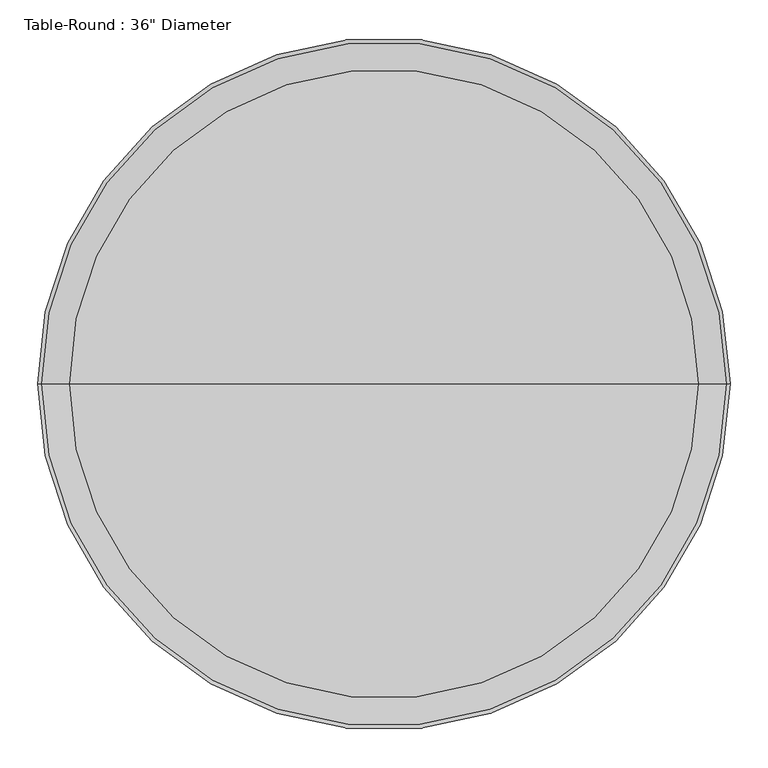
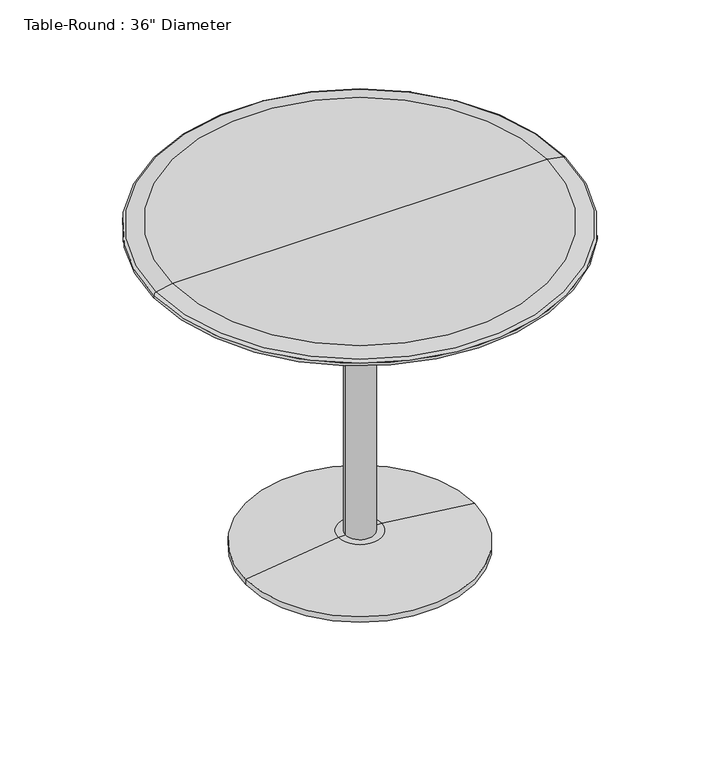
"""IFC4 building model written with IfcOpenShell, lengths in millimetres: furniture geometry."""

from ifc_helpers import new_model, si_unit, point, frame, origin, origin_2d, place, context, project, spatial, polyline, circle_curve, ellipse_curve, trimmed, segment, composite_curve, outline, extrude, source, transform, mapped, element, save
from ifc_brep_helpers import plane_surface, cylinder_surface, revolved_surface, advanced_brep


def furniture_f9efd34a(model_context):
    return source(origin(), model_context, "Body", "SolidModel", [
        extrude(outline(composite_curve([segment(trimmed(circle_curve(origin_2d(), 31.75), [point((-31.75, 0.0))], [point((31.75, 0.0))], False, "CARTESIAN"), True, "CONTINUOUS"), segment(trimmed(circle_curve(origin_2d(), 31.75), [point((31.75, 0.0))], [point((-31.75, 0.0))], False, "CARTESIAN"), True, "CONTINUOUS")], self_intersect=False)), frame((0.0, 0.0, 38.1), z_axis=(0.0, 0.0, 1.0), x_axis=(1.0, 0.0, 0.0)), (0.0, 0.0, 1.0), 704.85),
        advanced_brep(
        [(0.0, 0.0, 0.0), (-254.0, 0.0, 0.0), (254.0, 0.0, 0.0), (47.625, 0.0, 38.1), (-47.625, 0.0, 38.1), (0.0, 0.0, 38.1), (254.0, 0.0, 12.7), (-254.0, 0.0, 12.7)],
        [
            (0, 1),
            (1, 2, circle_curve(frame((0.0, 0.0, 0.0), z_axis=(0.0, 0.0, -1.0), x_axis=(-1.0, 0.0, 0.0)), 254.0)),
            (2, 0),
            (2, 1, circle_curve(frame((0.0, 0.0, 0.0), z_axis=(0.0, 0.0, -1.0), x_axis=(-1.0, 0.0, 0.0)), 254.0)),
            (3, 4, circle_curve(frame((0.0, 0.0, 38.1), z_axis=(0.0, 0.0, 1.0), x_axis=(-1.0, 0.0, 0.0)), 47.625)),
            (4, 5),
            (5, 3),
            (4, 3, circle_curve(frame((0.0, 0.0, 38.1), z_axis=(0.0, 0.0, 1.0), x_axis=(-1.0, 0.0, 0.0)), 47.625)),
            (6, 7, circle_curve(frame((0.0, 0.0, 12.7), z_axis=(0.0, 0.0, 1.0), x_axis=(-1.0, 0.0, 0.0)), 254.0)),
            (7, 4),
            (3, 6),
            (7, 6, circle_curve(frame((0.0, 0.0, 12.7), z_axis=(0.0, 0.0, 1.0), x_axis=(-1.0, 0.0, 0.0)), 254.0)),
            (1, 7),
            (6, 2),
        ],
        [
            plane_surface(frame((0.0, 0.0, 0.0), z_axis=(0.0, 0.0, -1.0), x_axis=(-1.0, 0.0, 0.0))),
            plane_surface(frame((0.0, 0.0, 38.1), z_axis=(0.0, 0.0, 1.0), x_axis=(-1.0, 0.0, 0.0))),
            revolved_surface(polyline([(-47.625, 0.0, 38.1), (-254.0, 0.0, 12.7)]), (0.0, 0.0, 215.9), (0.0, 0.0, -1.0)),
            cylinder_surface(frame((0.0, 0.0, 215.9), z_axis=(0.0, 0.0, -1.0), x_axis=(-1.0, 0.0, 0.0)), 254.0),
        ],
        [
            (0, [[1, 2, 3]]),
            (0, [[-3, 4, -1]]),
            (1, [[5, 6, 7]]),
            (1, [[8, -7, -6]]),
            (2, [[9, 10, -5, 11]]),
            (2, [[12, -11, -8, -10]]),
            (3, [[-2, 13, -9, 14]]),
            (3, [[-4, -14, -12, -13]]),
        ],
    ),
        advanced_brep(
        [(0.0, 0.0, 742.95), (-457.2, 0.0, 742.95), (457.2, 0.0, 742.95), (415.3011364, 0.0, 762.0), (-415.3011364, 0.0, 762.0), (0.0, 0.0, 762.0), (451.9526659, 0.0, 755.5373465), (-451.9526659, 0.0, 755.5373465), (457.2, 0.0, 749.2838172), (-457.2, 0.0, 749.2838172)],
        [
            (0, 1),
            (1, 2, circle_curve(frame((0.0, 0.0, 742.95), z_axis=(0.0, 0.0, -1.0), x_axis=(-1.0, 0.0, 0.0)), 457.2)),
            (2, 0),
            (2, 1, circle_curve(frame((0.0, 0.0, 742.95), z_axis=(0.0, 0.0, -1.0), x_axis=(-1.0, 0.0, 0.0)), 457.2)),
            (3, 4, circle_curve(frame((0.0, 0.0, 762.0), z_axis=(0.0, 0.0, 1.0), x_axis=(-1.0, 0.0, 0.0)), 415.3011364)),
            (4, 5),
            (5, 3),
            (4, 3, circle_curve(frame((0.0, 0.0, 762.0), z_axis=(0.0, 0.0, 1.0), x_axis=(-1.0, 0.0, 0.0)), 415.3011364)),
            (6, 7, circle_curve(frame((0.0, 0.0, 755.5373465), z_axis=(0.0, 0.0, 1.0), x_axis=(-1.0, 0.0, 0.0)), 451.9526659)),
            (7, 4),
            (3, 6),
            (7, 6, circle_curve(frame((0.0, 0.0, 755.5373465), z_axis=(0.0, 0.0, 1.0), x_axis=(-1.0, 0.0, 0.0)), 451.9526659)),
            (8, 9, circle_curve(frame((0.0, 0.0, 749.2838172), z_axis=(0.0, 0.0, 1.0), x_axis=(-1.0, 0.0, 0.0)), 457.2)),
            (9, 7, circle_curve(frame((-450.85, 0.0, 749.2838172), z_axis=(0.0, 1.0, 0.0), x_axis=(1.0, 0.0, 0.0)), 6.35)),
            (6, 8, circle_curve(frame((450.85, 0.0, 749.2838172), z_axis=(0.0, 1.0, 0.0), x_axis=(-1.0, 0.0, 0.0)), 6.35)),
            (9, 8, circle_curve(frame((0.0, 0.0, 749.2838172), z_axis=(0.0, 0.0, 1.0), x_axis=(-1.0, 0.0, 0.0)), 457.2)),
            (1, 9),
            (8, 2),
        ],
        [
            plane_surface(frame((0.0, 0.0, 742.95), z_axis=(0.0, 0.0, -1.0), x_axis=(-1.0, 0.0, 0.0))),
            plane_surface(frame((0.0, 0.0, 762.0), z_axis=(0.0, 0.0, 1.0), x_axis=(-1.0, 0.0, 0.0))),
            revolved_surface(polyline([(-415.3011364, 0.0, 762.0), (-451.9526659, 0.0, 755.5373465)]), (0.0, 0.0, 838.2), (0.0, 0.0, -1.0)),
            revolved_surface(trimmed(ellipse_curve(frame((-450.85, 0.0, 749.2838172), z_axis=(0.0, -1.0, 0.0), x_axis=(1.0, 0.0, 0.0)), 6.35, 6.35), [point((-451.9526659, 0.0, 755.5373465))], [point((-457.2, 0.0, 749.2838172))], True, "CARTESIAN"), (0.0, 0.0, 838.2), (0.0, 0.0, -1.0)),
            cylinder_surface(frame((0.0, 0.0, 838.2), z_axis=(0.0, 0.0, -1.0), x_axis=(-1.0, 0.0, 0.0)), 457.2),
        ],
        [
            (0, [[1, 2, 3]]),
            (0, [[-3, 4, -1]]),
            (1, [[5, 6, 7]]),
            (1, [[8, -7, -6]]),
            (2, [[9, 10, -5, 11]]),
            (2, [[12, -11, -8, -10]]),
            (3, [[13, 14, -9, 15]]),
            (3, [[16, -15, -12, -14]]),
            (4, [[-2, 17, -13, 18]]),
            (4, [[-4, -18, -16, -17]]),
        ],
    ),
    ])


if __name__ == "__main__":
    model = new_model("IFC4")
    model_context = context("Model", 3, world=origin())
    ifc_project = project(units=[si_unit("LENGTHUNIT", "METRE", prefix="MILLI")], contexts=[model_context])
    site = spatial("IfcSite", under=ifc_project)
    building = spatial("IfcBuilding", under=site)
    placement = place(None, origin())
    furniture_shape = furniture_f9efd34a(model_context)
    element("IfcFurniture", 1, ObjectType="Table-Round : 36\" Diameter", at=placement, inside=building, context=model_context, shape_type="MappedRepresentation", body=[
        mapped(furniture_shape, transform((0.0, 0.0, 0.0), x_axis=(1.0, 0.0, 0.0), y_axis=(0.0, 1.0, 0.0), z_axis=(0.0, 0.0, 1.0))),
    ])
    save(model, "model.ifc")

# Revit data of these elements
# Type "Table-Round : 36\" Diameter"
#   Assembly Code = "E2020200"
#   Base Radius = 0' - 10"
#   Height = 2' - 6"
#   Radius = 1' - 6"
#   Base Material = Steel, Chrome Plated
#   Top Material = Birch
#   Default Elevation = 0
# Element 1 (IfcFurniture, "Table-Round : 36\" Diameter")
#   Materials on its faces: "Steel, Chrome Plated", "Birch"
# Materials
#   "Steel, Chrome Plated": class "Metal", colour RGB 216 216 216, transparency 0, Description = "Chromiuim plated steel", Cost = 0
#   "Birch": class "Wood", colour RGB 224 178 126, transparency 0, Description = "Betula Alleghaniensis", Cost = 0
